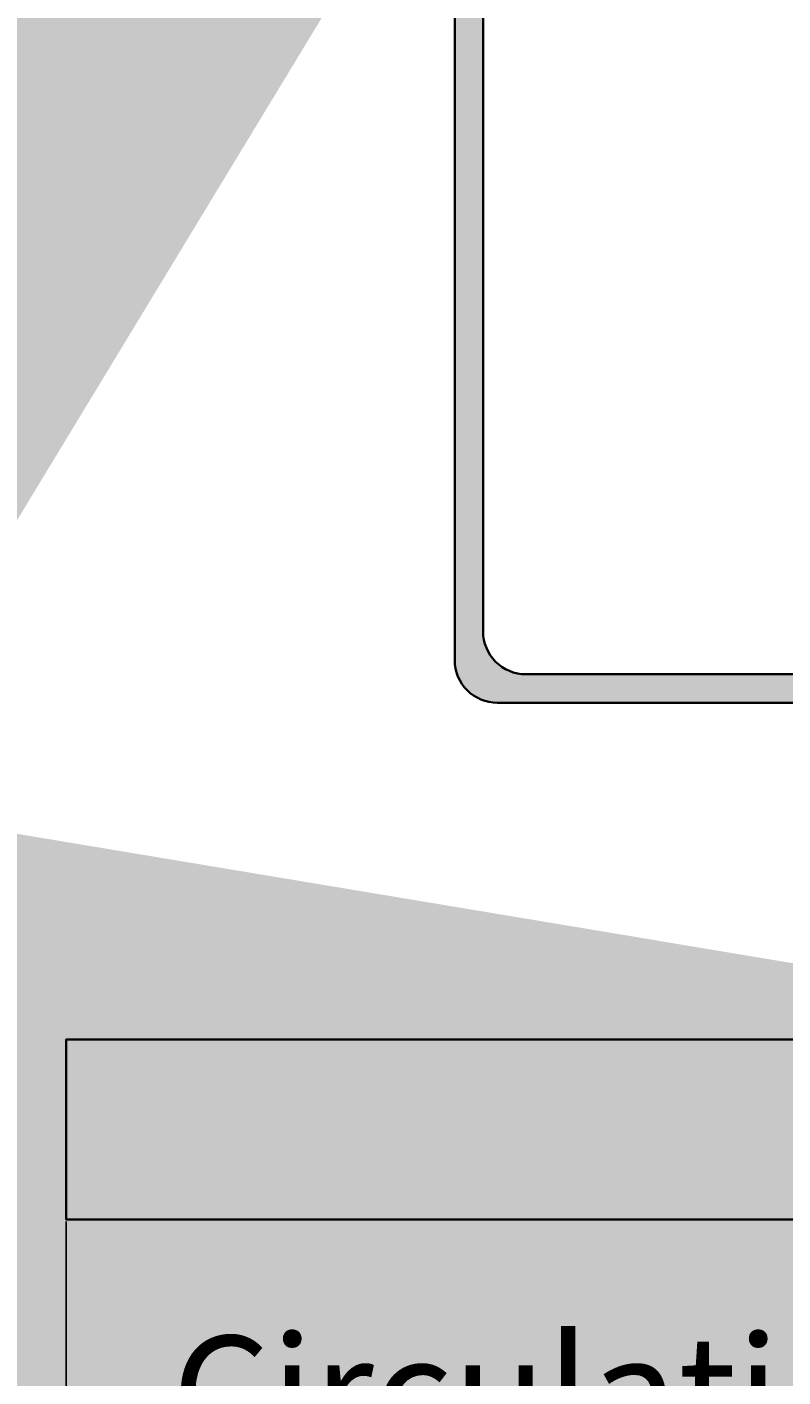
# Model space of a CAD drawing. Units: millimetres. Extents: x -22994 to 29398, y -19990 to 20176.
# Tile 9 of 135: x 5 to 32, y 5 to 52. Entities that reach past the tile are written whole.
import ezdxf
from ezdxf import colors
from ezdxf.entities.mleader import LeaderData, LeaderLine
from ezdxf.math import Vec2, Vec3

# ---------------------------------------------------------------- set-up
doc = ezdxf.new("R2010")
doc.units = ezdxf.units.MM
doc.header["$MEASUREMENT"] = 0
for name, color, linetype, lineweight in [('M-ANNO-TEXT', 7, 'Continuous', 25), ('M-DIMS', 2, 'Continuous', 18), ('M-EQPM-PATT', 7, 'Continuous', 18), ('M-PIPE', 7, 'Continuous', 35), ('S-FNDN', 7, 'Continuous', 35)]:
    doc.layers.add(name, color=color, linetype=linetype, lineweight=lineweight)
doc.styles.get("Standard").update_dxf_attribs({"font": 'arial.ttf'})
doc.dimstyles.get("Standard").update_dxf_attribs({"dimtxt": 0.18, "dimasz": 10000, "dimexe": 0.18, "dimexo": 0.0625, "dimgap": 0.09, "dimtad": 0, "dimtih": 1, "dimtoh": 1, "dimdec": 0, "dimzin": 0, "dimdsep": 46, "dimtxsty": 'Standard', "dimcen": 0.09, "dimadec": 0, "dimazin": 0, "dimtfac": 1, "dimtdec": 0, "dimtofl": 0, "dimtmove": 0, "dimatfit": 3, "dimfxl": 1, "dimtolj": 1, "dimtzin": 0, "dimlwd": 30, "dimarcsym": 0})

# ---------------------------------------------------------------- blocks, each defined once
blk = doc.blocks.new('*D2')
at = {"layer": 'Defpoints', "color": 0, "transparency": 16777216}
for p in [(6.677, 10.271), (290.852, 10.271), (290.852, -5.079)]:
    blk.add_point(p, dxfattribs=at)
at = {"layer": 'M-DIMS', "color": 0, "lineweight": -2, "transparency": 16777216}
for p, q in [((6.677, 10.209), (6.677, -5.259)), ((290.852, 10.209), (290.852, -5.259))]:
    blk.add_line(p, q, dxfattribs=at)
at = {"layer": 'M-DIMS', "color": 0, "lineweight": 30, "transparency": 16777216}
for p, q in [((-9993.323, -5.079), (-19993.323, -5.079)), ((10290.852, -5.079), (20290.852, -5.079))]:
    blk.add_line(p, q, dxfattribs=at)
at = {"layer": 'M-DIMS', "color": 0, "transparency": 16777216}
for points in [[(-9993.323, 1661.588), (-9993.323, -1671.745), (6.677, -5.079)], [(10290.852, 1661.588), (10290.852, -1671.745), (290.852, -5.079)]]:
    blk.add_solid(points, dxfattribs=at)
at = {"layer": 'M-DIMS', "color": 0, "transparency": 16777216, "insert": (148.765, -5.079), "char_height": 0.18, "attachment_point": 5}
blk.add_mtext('\\A1;284.2', dxfattribs=at)
blk = doc.blocks.new('*D3')
at = {"layer": 'Defpoints', "color": 0, "transparency": 16777216}
for p in [(110.265, 204.165), (110.265, 176.366), (95.833, 127.967)]:
    blk.add_point(p, dxfattribs=at)
at = {"layer": 'M-DIMS', "color": 0, "lineweight": 30, "transparency": 16777216}
for p, q in [((-9904.167, 204.165), (-19904.167, 204.165)), ((10110.265, 204.165), (20110.265, 204.165))]:
    blk.add_line(p, q, dxfattribs=at)
at = {"layer": 'M-DIMS', "color": 0, "lineweight": -2, "transparency": 16777216}
for p, q in [((95.833, 128.03), (95.833, 204.345)), ((110.265, 176.429), (110.265, 204.345))]:
    blk.add_line(p, q, dxfattribs=at)
at = {"layer": 'M-DIMS', "color": 0, "transparency": 16777216}
for points in [[(-9904.167, 1870.832), (-9904.167, -1462.501), (95.833, 204.165)], [(10110.265, 1870.832), (10110.265, -1462.501), (110.265, 204.165)]]:
    blk.add_solid(points, dxfattribs=at)
at = {"layer": 'M-DIMS', "color": 0, "transparency": 16777216, "insert": (103.049, 204.165), "char_height": 0.18, "attachment_point": 5}
blk.add_mtext('\\A1;14.432', dxfattribs=at)
blk = doc.blocks.new('*D4')
at = {"layer": 'Defpoints', "color": 0, "transparency": 16777216}
for p in [(116.265, 204.165), (110.265, 176.366), (116.265, 176.366)]:
    blk.add_point(p, dxfattribs=at)
at = {"layer": 'M-DIMS', "color": 0, "lineweight": 30, "transparency": 16777216}
for p, q in [((-9889.735, 204.165), (-19889.735, 204.165)), ((10116.265, 204.165), (20116.265, 204.165))]:
    blk.add_line(p, q, dxfattribs=at)
at = {"layer": 'M-DIMS', "color": 0, "lineweight": -2, "transparency": 16777216}
for p, q in [((110.265, 176.429), (110.265, 204.345)), ((116.265, 176.429), (116.265, 204.345))]:
    blk.add_line(p, q, dxfattribs=at)
at = {"layer": 'M-DIMS', "color": 0, "transparency": 16777216}
for points in [[(-9889.735, 1870.832), (-9889.735, -1462.501), (110.265, 204.165)], [(10116.265, 1870.832), (10116.265, -1462.501), (116.265, 204.165)]]:
    blk.add_solid(points, dxfattribs=at)
at = {"layer": 'M-DIMS', "color": 0, "transparency": 16777216, "insert": (113.265, 204.165), "char_height": 0.18, "attachment_point": 5}
blk.add_mtext('\\A1;6', dxfattribs=at)
blk = doc.blocks.new('*D5')
at = {"layer": 'Defpoints', "color": 0, "transparency": 16777216}
for p in [(181.265, 204.165), (116.265, 176.366), (181.265, 176.366)]:
    blk.add_point(p, dxfattribs=at)
at = {"layer": 'M-DIMS', "color": 0, "lineweight": 30, "transparency": 16777216}
for p, q in [((-9883.735, 204.165), (-19883.735, 204.165)), ((10181.265, 204.165), (20181.265, 204.165))]:
    blk.add_line(p, q, dxfattribs=at)
at = {"layer": 'M-DIMS', "color": 0, "lineweight": -2, "transparency": 16777216}
for p, q in [((116.265, 176.429), (116.265, 204.345)), ((181.265, 176.429), (181.265, 204.345))]:
    blk.add_line(p, q, dxfattribs=at)
at = {"layer": 'M-DIMS', "color": 0, "transparency": 16777216}
for points in [[(-9883.735, 1870.832), (-9883.735, -1462.501), (116.265, 204.165)], [(10181.265, 1870.832), (10181.265, -1462.501), (181.265, 204.165)]]:
    blk.add_solid(points, dxfattribs=at)
at = {"layer": 'M-DIMS', "color": 0, "transparency": 16777216, "insert": (148.765, 204.165), "char_height": 0.18, "attachment_point": 5}
blk.add_mtext('\\A1;65', dxfattribs=at)
blk = doc.blocks.new('*D6')
at = {"layer": 'Defpoints', "color": 0, "transparency": 16777216}
for p in [(187.265, 204.165), (181.265, 176.366), (187.265, 176.366)]:
    blk.add_point(p, dxfattribs=at)
at = {"layer": 'M-DIMS', "color": 0, "lineweight": 30, "transparency": 16777216}
for p, q in [((-9818.735, 204.165), (-19818.735, 204.165)), ((10187.265, 204.165), (20187.265, 204.165))]:
    blk.add_line(p, q, dxfattribs=at)
at = {"layer": 'M-DIMS', "color": 0, "lineweight": -2, "transparency": 16777216}
for p, q in [((181.265, 176.429), (181.265, 204.345)), ((187.265, 176.429), (187.265, 204.345))]:
    blk.add_line(p, q, dxfattribs=at)
at = {"layer": 'M-DIMS', "color": 0, "transparency": 16777216}
for points in [[(-9818.735, 1870.832), (-9818.735, -1462.501), (181.265, 204.165)], [(10187.265, 1870.832), (10187.265, -1462.501), (187.265, 204.165)]]:
    blk.add_solid(points, dxfattribs=at)
at = {"layer": 'M-DIMS', "color": 0, "transparency": 16777216, "insert": (184.265, 204.165), "char_height": 0.18, "attachment_point": 5}
blk.add_mtext('\\A1;6', dxfattribs=at)
blk = doc.blocks.new('*D7')
at = {"layer": 'Defpoints', "color": 0, "transparency": 16777216}
for p in [(201.697, 204.165), (187.265, 176.366), (201.697, 127.967)]:
    blk.add_point(p, dxfattribs=at)
at = {"layer": 'M-DIMS', "color": 0, "lineweight": 30, "transparency": 16777216}
for p, q in [((-9812.735, 204.165), (-19812.735, 204.165)), ((10201.697, 204.165), (20201.697, 204.165))]:
    blk.add_line(p, q, dxfattribs=at)
at = {"layer": 'M-DIMS', "color": 0, "lineweight": -2, "transparency": 16777216}
for p, q in [((187.265, 176.429), (187.265, 204.345)), ((201.697, 128.03), (201.697, 204.345))]:
    blk.add_line(p, q, dxfattribs=at)
at = {"layer": 'M-DIMS', "color": 0, "transparency": 16777216}
for points in [[(-9812.735, 1870.832), (-9812.735, -1462.501), (187.265, 204.165)], [(10201.697, 1870.832), (10201.697, -1462.501), (201.697, 204.165)]]:
    blk.add_solid(points, dxfattribs=at)
at = {"layer": 'M-DIMS', "color": 0, "transparency": 16777216, "insert": (194.481, 204.165), "char_height": 0.18, "attachment_point": 5}
blk.add_mtext('\\A1;14.432', dxfattribs=at)
blk = doc.blocks.new('*D8')
at = {"layer": 'Defpoints', "color": 0, "transparency": 16777216}
for p in [(227.648, 204.165), (227.648, 146.73), (201.697, 127.967)]:
    blk.add_point(p, dxfattribs=at)
at = {"layer": 'M-DIMS', "color": 0, "lineweight": 30, "transparency": 16777216}
for p, q in [((-9798.303, 204.165), (-19798.303, 204.165)), ((10227.648, 204.165), (20227.648, 204.165))]:
    blk.add_line(p, q, dxfattribs=at)
at = {"layer": 'M-DIMS', "color": 0, "lineweight": -2, "transparency": 16777216}
for p, q in [((201.697, 128.03), (201.697, 204.345)), ((227.648, 146.792), (227.648, 204.345))]:
    blk.add_line(p, q, dxfattribs=at)
at = {"layer": 'M-DIMS', "color": 0, "transparency": 16777216}
for points in [[(-9798.303, 1870.832), (-9798.303, -1462.501), (201.697, 204.165)], [(10227.648, 1870.832), (10227.648, -1462.501), (227.648, 204.165)]]:
    blk.add_solid(points, dxfattribs=at)
at = {"layer": 'M-DIMS', "color": 0, "transparency": 16777216, "insert": (214.673, 204.165), "char_height": 0.18, "attachment_point": 5}
blk.add_mtext('\\A1;25.95', dxfattribs=at)
blk = doc.blocks.new('*D9')
at = {"layer": 'Defpoints', "color": 0, "transparency": 16777216}
for p in [(187.265, 176.366), (306.202, 176.366), (290.852, 10.271)]:
    blk.add_point(p, dxfattribs=at)
at = {"layer": 'M-DIMS', "color": 0, "lineweight": 30, "transparency": 16777216}
for p, q in [((306.202, 10176.366), (306.202, 20176.366)), ((306.202, -9989.729), (306.202, -19989.729))]:
    blk.add_line(p, q, dxfattribs=at)
at = {"layer": 'M-DIMS', "color": 0, "lineweight": -2, "transparency": 16777216}
for p, q in [((187.327, 176.366), (306.382, 176.366)), ((290.915, 10.271), (306.382, 10.271))]:
    blk.add_line(p, q, dxfattribs=at)
at = {"layer": 'M-DIMS', "color": 0, "transparency": 16777216}
for points in [[(-1360.465, 10176.366), (1972.869, 10176.366), (306.202, 176.366)], [(-1360.465, -9989.729), (1972.869, -9989.729), (306.202, 10.271)]]:
    blk.add_solid(points, dxfattribs=at)
at = {"layer": 'M-DIMS', "color": 0, "transparency": 16777216, "insert": (306.202, 93.319), "char_height": 0.18, "attachment_point": 5}
blk.add_mtext('\\A1;166.1', dxfattribs=at)
blk = doc.blocks.new('*D10')
at = {"layer": 'Defpoints', "color": 0, "transparency": 16777216}
for p in [(125.65, 136.071), (133.346, 136.071), (133.346, -5.079)]:
    blk.add_point(p, dxfattribs=at)
at = {"layer": 'M-DIMS', "color": 0, "lineweight": -2, "transparency": 16777216}
for p, q in [((125.65, 136.009), (125.65, -5.259)), ((133.346, 136.009), (133.346, -5.259))]:
    blk.add_line(p, q, dxfattribs=at)
at = {"layer": 'M-DIMS', "color": 0, "lineweight": 30, "transparency": 16777216}
for p, q in [((-9874.35, -5.079), (-19874.35, -5.079)), ((10133.346, -5.079), (20133.346, -5.079))]:
    blk.add_line(p, q, dxfattribs=at)
at = {"layer": 'M-DIMS', "color": 0, "transparency": 16777216}
for points in [[(-9874.35, 1661.588), (-9874.35, -1671.745), (125.65, -5.079)], [(10133.346, 1661.588), (10133.346, -1671.745), (133.346, -5.079)]]:
    blk.add_solid(points, dxfattribs=at)
at = {"layer": 'M-DIMS', "color": 0, "transparency": 16777216, "insert": (129.498, -5.079), "char_height": 0.18, "attachment_point": 5}
blk.add_mtext('\\A1;7.696', dxfattribs=at)
blk = doc.blocks.new('*D11')
at = {"layer": 'Defpoints', "color": 0, "transparency": 16777216}
for p in [(133.346, 136.071), (135.65, 136.071), (135.65, -5.079)]:
    blk.add_point(p, dxfattribs=at)
at = {"layer": 'M-DIMS', "color": 0, "lineweight": -2, "transparency": 16777216}
for p, q in [((133.346, 136.009), (133.346, -5.259)), ((135.65, 136.009), (135.65, -5.259))]:
    blk.add_line(p, q, dxfattribs=at)
at = {"layer": 'M-DIMS', "color": 0, "lineweight": 30, "transparency": 16777216}
for p, q in [((-9866.654, -5.079), (-19866.654, -5.079)), ((10135.65, -5.079), (20135.65, -5.079))]:
    blk.add_line(p, q, dxfattribs=at)
at = {"layer": 'M-DIMS', "color": 0, "transparency": 16777216}
for points in [[(-9866.654, 1661.588), (-9866.654, -1671.745), (133.346, -5.079)], [(10135.65, 1661.588), (10135.65, -1671.745), (135.65, -5.079)]]:
    blk.add_solid(points, dxfattribs=at)
at = {"layer": 'M-DIMS', "color": 0, "transparency": 16777216, "insert": (134.498, -5.079), "char_height": 0.18, "attachment_point": 5}
blk.add_mtext('\\A1;2.304', dxfattribs=at)
blk = doc.blocks.new('*D12')
at = {"layer": 'Defpoints', "color": 0, "transparency": 16777216}
for p in [(135.65, 136.071), (145.65, 136.071), (145.65, -5.079)]:
    blk.add_point(p, dxfattribs=at)
at = {"layer": 'M-DIMS', "color": 0, "lineweight": -2, "transparency": 16777216}
for p, q in [((135.65, 136.009), (135.65, -5.259)), ((145.65, 136.009), (145.65, -5.259))]:
    blk.add_line(p, q, dxfattribs=at)
at = {"layer": 'M-DIMS', "color": 0, "lineweight": 30, "transparency": 16777216}
for p, q in [((-9864.35, -5.079), (-19864.35, -5.079)), ((10145.65, -5.079), (20145.65, -5.079))]:
    blk.add_line(p, q, dxfattribs=at)
at = {"layer": 'M-DIMS', "color": 0, "transparency": 16777216}
for points in [[(-9864.35, 1661.588), (-9864.35, -1671.745), (135.65, -5.079)], [(10145.65, 1661.588), (10145.65, -1671.745), (145.65, -5.079)]]:
    blk.add_solid(points, dxfattribs=at)
at = {"layer": 'M-DIMS', "color": 0, "transparency": 16777216, "insert": (140.65, -5.079), "char_height": 0.18, "attachment_point": 5}
blk.add_mtext('\\A1;10', dxfattribs=at)
blk = doc.blocks.new('*D13')
at = {"layer": 'Defpoints', "color": 0, "transparency": 16777216}
for p in [(145.65, 136.071), (155.65, 136.071), (155.65, -5.079)]:
    blk.add_point(p, dxfattribs=at)
at = {"layer": 'M-DIMS', "color": 0, "lineweight": -2, "transparency": 16777216}
for p, q in [((145.65, 136.009), (145.65, -5.259)), ((155.65, 136.009), (155.65, -5.259))]:
    blk.add_line(p, q, dxfattribs=at)
at = {"layer": 'M-DIMS', "color": 0, "lineweight": 30, "transparency": 16777216}
for p, q in [((-9854.35, -5.079), (-19854.35, -5.079)), ((10155.65, -5.079), (20155.65, -5.079))]:
    blk.add_line(p, q, dxfattribs=at)
at = {"layer": 'M-DIMS', "color": 0, "transparency": 16777216}
for points in [[(-9854.35, 1661.588), (-9854.35, -1671.745), (145.65, -5.079)], [(10155.65, 1661.588), (10155.65, -1671.745), (155.65, -5.079)]]:
    blk.add_solid(points, dxfattribs=at)
at = {"layer": 'M-DIMS', "color": 0, "transparency": 16777216, "insert": (150.65, -5.079), "char_height": 0.18, "attachment_point": 5}
blk.add_mtext('\\A1;10', dxfattribs=at)
blk = doc.blocks.new('*D14')
at = {"layer": 'Defpoints', "color": 0, "transparency": 16777216}
for p in [(155.65, 136.071), (165.65, 136.071), (165.65, -5.079)]:
    blk.add_point(p, dxfattribs=at)
at = {"layer": 'M-DIMS', "color": 0, "lineweight": -2, "transparency": 16777216}
for p, q in [((155.65, 136.009), (155.65, -5.259)), ((165.65, 136.009), (165.65, -5.259))]:
    blk.add_line(p, q, dxfattribs=at)
at = {"layer": 'M-DIMS', "color": 0, "lineweight": 30, "transparency": 16777216}
for p, q in [((-9844.35, -5.079), (-19844.35, -5.079)), ((10165.65, -5.079), (20165.65, -5.079))]:
    blk.add_line(p, q, dxfattribs=at)
at = {"layer": 'M-DIMS', "color": 0, "transparency": 16777216}
for points in [[(-9844.35, 1661.588), (-9844.35, -1671.745), (155.65, -5.079)], [(10165.65, 1661.588), (10165.65, -1671.745), (165.65, -5.079)]]:
    blk.add_solid(points, dxfattribs=at)
at = {"layer": 'M-DIMS', "color": 0, "transparency": 16777216, "insert": (160.65, -5.079), "char_height": 0.18, "attachment_point": 5}
blk.add_mtext('\\A1;10', dxfattribs=at)
blk = doc.blocks.new('*D15')
at = {"layer": 'Defpoints', "color": 0, "transparency": 16777216}
for p in [(173.346, 154.788), (173.346, 136.071), (306.202, 136.071)]:
    blk.add_point(p, dxfattribs=at)
at = {"layer": 'M-DIMS', "color": 0, "lineweight": 30, "transparency": 16777216}
for p, q in [((306.202, 10154.788), (306.202, 20154.788)), ((306.202, -9863.929), (306.202, -19863.929))]:
    blk.add_line(p, q, dxfattribs=at)
at = {"layer": 'M-DIMS', "color": 0, "lineweight": -2, "transparency": 16777216}
for p, q in [((173.408, 154.788), (306.382, 154.788)), ((173.408, 136.071), (306.382, 136.071))]:
    blk.add_line(p, q, dxfattribs=at)
at = {"layer": 'M-DIMS', "color": 0, "transparency": 16777216}
for points in [[(-1360.465, 10154.788), (1972.869, 10154.788), (306.202, 154.788)], [(-1360.465, -9863.929), (1972.869, -9863.929), (306.202, 136.071)]]:
    blk.add_solid(points, dxfattribs=at)
at = {"layer": 'M-DIMS', "color": 0, "transparency": 16777216, "insert": (306.202, 145.43), "char_height": 0.18, "attachment_point": 5}
blk.add_mtext('\\A1;18.717', dxfattribs=at)
blk = doc.blocks.new('*D16')
at = {"layer": 'Defpoints', "color": 0, "transparency": 16777216}
for p in [(120.17, 204.165), (110.466, 48.035), (120.17, 48.035)]:
    blk.add_point(p, dxfattribs=at)
at = {"layer": 'M-DIMS', "color": 0, "lineweight": 30, "transparency": 16777216}
for p, q in [((-9889.534, 204.165), (-19889.534, 204.165)), ((10120.17, 204.165), (20120.17, 204.165))]:
    blk.add_line(p, q, dxfattribs=at)
at = {"layer": 'M-DIMS', "color": 0, "lineweight": -2, "transparency": 16777216}
for p, q in [((110.466, 48.097), (110.466, 204.345)), ((120.17, 48.097), (120.17, 204.345))]:
    blk.add_line(p, q, dxfattribs=at)
at = {"layer": 'M-DIMS', "color": 0, "transparency": 16777216}
for points in [[(-9889.534, 1870.832), (-9889.534, -1462.501), (110.466, 204.165)], [(10120.17, 1870.832), (10120.17, -1462.501), (120.17, 204.165)]]:
    blk.add_solid(points, dxfattribs=at)
at = {"layer": 'M-DIMS', "color": 0, "transparency": 16777216, "insert": (115.318, 204.165), "char_height": 0.18, "attachment_point": 5}
blk.add_mtext('\\A1;9.704', dxfattribs=at)
blk = doc.blocks.new('*D17')
at = {"layer": 'Defpoints', "color": 0, "transparency": 16777216}
for p in [(126.17, 204.165), (120.17, 48.035), (126.17, 48.035)]:
    blk.add_point(p, dxfattribs=at)
at = {"layer": 'M-DIMS', "color": 0, "lineweight": 30, "transparency": 16777216}
for p, q in [((-9879.83, 204.165), (-19879.83, 204.165)), ((10126.17, 204.165), (20126.17, 204.165))]:
    blk.add_line(p, q, dxfattribs=at)
at = {"layer": 'M-DIMS', "color": 0, "lineweight": -2, "transparency": 16777216}
for p, q in [((120.17, 48.097), (120.17, 204.345)), ((126.17, 48.097), (126.17, 204.345))]:
    blk.add_line(p, q, dxfattribs=at)
at = {"layer": 'M-DIMS', "color": 0, "transparency": 16777216}
for points in [[(-9879.83, 1870.832), (-9879.83, -1462.501), (120.17, 204.165)], [(10126.17, 1870.832), (10126.17, -1462.501), (126.17, 204.165)]]:
    blk.add_solid(points, dxfattribs=at)
at = {"layer": 'M-DIMS', "color": 0, "transparency": 16777216, "insert": (123.17, 204.165), "char_height": 0.18, "attachment_point": 5}
blk.add_mtext('\\A1;6', dxfattribs=at)
blk = doc.blocks.new('*D18')
at = {"layer": 'Defpoints', "color": 0, "transparency": 16777216}
for p in [(132.17, 204.165), (126.17, 48.035), (132.17, 48.035)]:
    blk.add_point(p, dxfattribs=at)
at = {"layer": 'M-DIMS', "color": 0, "lineweight": 30, "transparency": 16777216}
for p, q in [((-9873.83, 204.165), (-19873.83, 204.165)), ((10132.17, 204.165), (20132.17, 204.165))]:
    blk.add_line(p, q, dxfattribs=at)
at = {"layer": 'M-DIMS', "color": 0, "lineweight": -2, "transparency": 16777216}
for p, q in [((126.17, 48.097), (126.17, 204.345)), ((132.17, 48.097), (132.17, 204.345))]:
    blk.add_line(p, q, dxfattribs=at)
at = {"layer": 'M-DIMS', "color": 0, "transparency": 16777216}
for points in [[(-9873.83, 1870.832), (-9873.83, -1462.501), (126.17, 204.165)], [(10132.17, 1870.832), (10132.17, -1462.501), (132.17, 204.165)]]:
    blk.add_solid(points, dxfattribs=at)
at = {"layer": 'M-DIMS', "color": 0, "transparency": 16777216, "insert": (129.17, 204.165), "char_height": 0.18, "attachment_point": 5}
blk.add_mtext('\\A1;6', dxfattribs=at)
blk = doc.blocks.new('*D19')
at = {"layer": 'Defpoints', "color": 0, "transparency": 16777216}
for p in [(138.17, 204.165), (132.17, 48.035), (138.17, 48.035)]:
    blk.add_point(p, dxfattribs=at)
at = {"layer": 'M-DIMS', "color": 0, "lineweight": 30, "transparency": 16777216}
for p, q in [((-9867.83, 204.165), (-19867.83, 204.165)), ((10138.17, 204.165), (20138.17, 204.165))]:
    blk.add_line(p, q, dxfattribs=at)
at = {"layer": 'M-DIMS', "color": 0, "lineweight": -2, "transparency": 16777216}
for p, q in [((132.17, 48.097), (132.17, 204.345)), ((138.17, 48.097), (138.17, 204.345))]:
    blk.add_line(p, q, dxfattribs=at)
at = {"layer": 'M-DIMS', "color": 0, "transparency": 16777216}
for points in [[(-9867.83, 1870.832), (-9867.83, -1462.501), (132.17, 204.165)], [(10138.17, 1870.832), (10138.17, -1462.501), (138.17, 204.165)]]:
    blk.add_solid(points, dxfattribs=at)
at = {"layer": 'M-DIMS', "color": 0, "transparency": 16777216, "insert": (135.17, 204.165), "char_height": 0.18, "attachment_point": 5}
blk.add_mtext('\\A1;6', dxfattribs=at)
blk = doc.blocks.new('*D20')
at = {"layer": 'Defpoints', "color": 0, "transparency": 16777216}
for p in [(144.17, 204.165), (138.17, 48.035), (144.17, 48.035)]:
    blk.add_point(p, dxfattribs=at)
at = {"layer": 'M-DIMS', "color": 0, "lineweight": 30, "transparency": 16777216}
for p, q in [((-9861.83, 204.165), (-19861.83, 204.165)), ((10144.17, 204.165), (20144.17, 204.165))]:
    blk.add_line(p, q, dxfattribs=at)
at = {"layer": 'M-DIMS', "color": 0, "lineweight": -2, "transparency": 16777216}
for p, q in [((138.17, 48.097), (138.17, 204.345)), ((144.17, 48.097), (144.17, 204.345))]:
    blk.add_line(p, q, dxfattribs=at)
at = {"layer": 'M-DIMS', "color": 0, "transparency": 16777216}
for points in [[(-9861.83, 1870.832), (-9861.83, -1462.501), (138.17, 204.165)], [(10144.17, 1870.832), (10144.17, -1462.501), (144.17, 204.165)]]:
    blk.add_solid(points, dxfattribs=at)
at = {"layer": 'M-DIMS', "color": 0, "transparency": 16777216, "insert": (141.17, 204.165), "char_height": 0.18, "attachment_point": 5}
blk.add_mtext('\\A1;6', dxfattribs=at)
blk = doc.blocks.new('*D21')
at = {"layer": 'Defpoints', "color": 0, "transparency": 16777216}
for p in [(149.116, 204.165), (144.17, 48.035), (149.116, 48.035)]:
    blk.add_point(p, dxfattribs=at)
at = {"layer": 'M-DIMS', "color": 0, "lineweight": 30, "transparency": 16777216}
for p, q in [((-9855.83, 204.165), (-19855.83, 204.165)), ((10149.116, 204.165), (20149.116, 204.165))]:
    blk.add_line(p, q, dxfattribs=at)
at = {"layer": 'M-DIMS', "color": 0, "lineweight": -2, "transparency": 16777216}
for p, q in [((144.17, 48.097), (144.17, 204.345)), ((149.116, 48.097), (149.116, 204.345))]:
    blk.add_line(p, q, dxfattribs=at)
at = {"layer": 'M-DIMS', "color": 0, "transparency": 16777216}
for points in [[(-9855.83, 1870.832), (-9855.83, -1462.501), (144.17, 204.165)], [(10149.116, 1870.832), (10149.116, -1462.501), (149.116, 204.165)]]:
    blk.add_solid(points, dxfattribs=at)
at = {"layer": 'M-DIMS', "color": 0, "transparency": 16777216, "insert": (146.643, 204.165), "char_height": 0.18, "attachment_point": 5}
blk.add_mtext('\\A1;4.945', dxfattribs=at)
blk = doc.blocks.new('*D22')
at = {"layer": 'Defpoints', "color": 0, "transparency": 16777216}
for p in [(149.116, 30.99), (155.116, 30.99), (155.116, -5.079)]:
    blk.add_point(p, dxfattribs=at)
at = {"layer": 'M-DIMS', "color": 0, "lineweight": -2, "transparency": 16777216}
for p, q in [((149.116, 30.927), (149.116, -5.259)), ((155.116, 30.927), (155.116, -5.259))]:
    blk.add_line(p, q, dxfattribs=at)
at = {"layer": 'M-DIMS', "color": 0, "lineweight": 30, "transparency": 16777216}
for p, q in [((-9850.884, -5.079), (-19850.884, -5.079)), ((10155.116, -5.079), (20155.116, -5.079))]:
    blk.add_line(p, q, dxfattribs=at)
at = {"layer": 'M-DIMS', "color": 0, "transparency": 16777216}
for points in [[(-9850.884, 1661.588), (-9850.884, -1671.745), (149.116, -5.079)], [(10155.116, 1661.588), (10155.116, -1671.745), (155.116, -5.079)]]:
    blk.add_solid(points, dxfattribs=at)
at = {"layer": 'M-DIMS', "color": 0, "transparency": 16777216, "insert": (152.116, -5.079), "char_height": 0.18, "attachment_point": 5}
blk.add_mtext('\\A1;6', dxfattribs=at)
blk = doc.blocks.new('*D23')
at = {"layer": 'Defpoints', "color": 0, "transparency": 16777216}
for p in [(155.116, 30.99), (161.116, 30.99), (161.116, -5.079)]:
    blk.add_point(p, dxfattribs=at)
at = {"layer": 'M-DIMS', "color": 0, "lineweight": -2, "transparency": 16777216}
for p, q in [((155.116, 30.927), (155.116, -5.259)), ((161.116, 30.927), (161.116, -5.259))]:
    blk.add_line(p, q, dxfattribs=at)
at = {"layer": 'M-DIMS', "color": 0, "lineweight": 30, "transparency": 16777216}
for p, q in [((-9844.884, -5.079), (-19844.884, -5.079)), ((10161.116, -5.079), (20161.116, -5.079))]:
    blk.add_line(p, q, dxfattribs=at)
at = {"layer": 'M-DIMS', "color": 0, "transparency": 16777216}
for points in [[(-9844.884, 1661.588), (-9844.884, -1671.745), (155.116, -5.079)], [(10161.116, 1661.588), (10161.116, -1671.745), (161.116, -5.079)]]:
    blk.add_solid(points, dxfattribs=at)
at = {"layer": 'M-DIMS', "color": 0, "transparency": 16777216, "insert": (158.116, -5.079), "char_height": 0.18, "attachment_point": 5}
blk.add_mtext('\\A1;6', dxfattribs=at)
blk = doc.blocks.new('*D24')
at = {"layer": 'Defpoints', "color": 0, "transparency": 16777216}
for p in [(161.116, 30.99), (166.439, 30.99), (166.439, -5.079)]:
    blk.add_point(p, dxfattribs=at)
at = {"layer": 'M-DIMS', "color": 0, "lineweight": -2, "transparency": 16777216}
for p, q in [((161.116, 30.927), (161.116, -5.259)), ((166.439, 30.927), (166.439, -5.259))]:
    blk.add_line(p, q, dxfattribs=at)
at = {"layer": 'M-DIMS', "color": 0, "lineweight": 30, "transparency": 16777216}
for p, q in [((-9838.884, -5.079), (-19838.884, -5.079)), ((10166.439, -5.079), (20166.439, -5.079))]:
    blk.add_line(p, q, dxfattribs=at)
at = {"layer": 'M-DIMS', "color": 0, "transparency": 16777216}
for points in [[(-9838.884, 1661.588), (-9838.884, -1671.745), (161.116, -5.079)], [(10166.439, 1661.588), (10166.439, -1671.745), (166.439, -5.079)]]:
    blk.add_solid(points, dxfattribs=at)
at = {"layer": 'M-DIMS', "color": 0, "transparency": 16777216, "insert": (163.777, -5.079), "char_height": 0.18, "attachment_point": 5}
blk.add_mtext('\\A1;5.323', dxfattribs=at)
blk = doc.blocks.new('*D25')
at = {"layer": 'Defpoints', "color": 0, "transparency": 16777216}
for p in [(166.439, 30.99), (172.439, 30.99), (172.439, -5.079)]:
    blk.add_point(p, dxfattribs=at)
at = {"layer": 'M-DIMS', "color": 0, "lineweight": -2, "transparency": 16777216}
for p, q in [((166.439, 30.927), (166.439, -5.259)), ((172.439, 30.927), (172.439, -5.259))]:
    blk.add_line(p, q, dxfattribs=at)
at = {"layer": 'M-DIMS', "color": 0, "lineweight": 30, "transparency": 16777216}
for p, q in [((-9833.561, -5.079), (-19833.561, -5.079)), ((10172.439, -5.079), (20172.439, -5.079))]:
    blk.add_line(p, q, dxfattribs=at)
at = {"layer": 'M-DIMS', "color": 0, "transparency": 16777216}
for points in [[(-9833.561, 1661.588), (-9833.561, -1671.745), (166.439, -5.079)], [(10172.439, 1661.588), (10172.439, -1671.745), (172.439, -5.079)]]:
    blk.add_solid(points, dxfattribs=at)
at = {"layer": 'M-DIMS', "color": 0, "transparency": 16777216, "insert": (169.439, -5.079), "char_height": 0.18, "attachment_point": 5}
blk.add_mtext('\\A1;6', dxfattribs=at)
blk = doc.blocks.new('*D26')
at = {"layer": 'Defpoints', "color": 0, "transparency": 16777216}
for p in [(172.439, 30.99), (178.439, 30.99), (178.439, -5.079)]:
    blk.add_point(p, dxfattribs=at)
at = {"layer": 'M-DIMS', "color": 0, "lineweight": -2, "transparency": 16777216}
for p, q in [((172.439, 30.927), (172.439, -5.259)), ((178.439, 30.927), (178.439, -5.259))]:
    blk.add_line(p, q, dxfattribs=at)
at = {"layer": 'M-DIMS', "color": 0, "lineweight": 30, "transparency": 16777216}
for p, q in [((-9827.561, -5.079), (-19827.561, -5.079)), ((10178.439, -5.079), (20178.439, -5.079))]:
    blk.add_line(p, q, dxfattribs=at)
at = {"layer": 'M-DIMS', "color": 0, "transparency": 16777216}
for points in [[(-9827.561, 1661.588), (-9827.561, -1671.745), (172.439, -5.079)], [(10178.439, 1661.588), (10178.439, -1671.745), (178.439, -5.079)]]:
    blk.add_solid(points, dxfattribs=at)
at = {"layer": 'M-DIMS', "color": 0, "transparency": 16777216, "insert": (175.439, -5.079), "char_height": 0.18, "attachment_point": 5}
blk.add_mtext('\\A1;6', dxfattribs=at)
blk = doc.blocks.new('*D27')
at = {"layer": 'Defpoints', "color": 0, "transparency": 16777216}
for p in [(178.439, 30.99), (188.117, 30.99), (188.117, -5.079)]:
    blk.add_point(p, dxfattribs=at)
at = {"layer": 'M-DIMS', "color": 0, "lineweight": -2, "transparency": 16777216}
for p, q in [((178.439, 30.927), (178.439, -5.259)), ((188.117, 30.927), (188.117, -5.259))]:
    blk.add_line(p, q, dxfattribs=at)
at = {"layer": 'M-DIMS', "color": 0, "lineweight": 30, "transparency": 16777216}
for p, q in [((-9821.561, -5.079), (-19821.561, -5.079)), ((10188.117, -5.079), (20188.117, -5.079))]:
    blk.add_line(p, q, dxfattribs=at)
at = {"layer": 'M-DIMS', "color": 0, "transparency": 16777216}
for points in [[(-9821.561, 1661.588), (-9821.561, -1671.745), (178.439, -5.079)], [(10188.117, 1661.588), (10188.117, -1671.745), (188.117, -5.079)]]:
    blk.add_solid(points, dxfattribs=at)
at = {"layer": 'M-DIMS', "color": 0, "transparency": 16777216, "insert": (183.278, -5.079), "char_height": 0.18, "attachment_point": 5}
blk.add_mtext('\\A1;9.679', dxfattribs=at)
blk = doc.blocks.new('*D28')
at = {"layer": 'Defpoints', "color": 0, "transparency": 16777216}
for p in [(188.117, 48.035), (306.202, 48.035), (188.117, 30.99)]:
    blk.add_point(p, dxfattribs=at)
at = {"layer": 'M-DIMS', "color": 0, "lineweight": 30, "transparency": 16777216}
for p, q in [((306.202, 10048.035), (306.202, 20048.035)), ((306.202, -9969.01), (306.202, -19969.01))]:
    blk.add_line(p, q, dxfattribs=at)
at = {"layer": 'M-DIMS', "color": 0, "lineweight": -2, "transparency": 16777216}
for p, q in [((188.18, 48.035), (306.382, 48.035)), ((188.18, 30.99), (306.382, 30.99))]:
    blk.add_line(p, q, dxfattribs=at)
at = {"layer": 'M-DIMS', "color": 0, "transparency": 16777216}
for points in [[(-1360.465, 10048.035), (1972.869, 10048.035), (306.202, 48.035)], [(-1360.465, -9969.01), (1972.869, -9969.01), (306.202, 30.99)]]:
    blk.add_solid(points, dxfattribs=at)
at = {"layer": 'M-DIMS', "color": 0, "transparency": 16777216, "insert": (306.202, 39.512), "char_height": 0.18, "attachment_point": 5}
blk.add_mtext('\\A1;17.045', dxfattribs=at)
blk = doc.blocks.new('*D32')
at = {"layer": 'Defpoints', "color": 0, "transparency": 16777216}
for p in [(57.164, 118.614), (52.413, 113.093)]:
    blk.add_point(p, dxfattribs=at)
at = {"layer": 'M-DIMS', "color": 0, "lineweight": -2, "transparency": 16777216}
for p, q in [((57.164, 118.524), (57.164, 118.704)), ((57.074, 118.614), (57.254, 118.614))]:
    blk.add_line(p, q, dxfattribs=at)
at = {"layer": 'M-DIMS', "color": 0, "lineweight": 30, "transparency": 16777216}
for p, q in [((-12992.534, -15047.031), (-6470.06, -7466.969)), ((-22992.534, -15047.031), (-12992.534, -15047.031))]:
    blk.add_line(p, q, dxfattribs=at)
at = {"layer": 'M-DIMS', "color": 0, "transparency": 16777216}
blk.add_solid([(-7733.404, -6379.89), (-5206.717, -8554.048), (52.413, 113.093)], dxfattribs=at)
at = {"layer": 'M-DIMS', "color": 0, "transparency": 16777216, "insert": (-22993.208, -15047.031), "char_height": 0.18, "attachment_point": 5}
blk.add_mtext('\\A1;2X R7.284', dxfattribs=at)
blk = doc.blocks.new('*D36')
at = {"layer": 'Defpoints', "color": 0, "transparency": 16777216}
for p in [(46.39, 31.303), (46.387, 26.593)]:
    blk.add_point(p, dxfattribs=at)
at = {"layer": 'M-DIMS', "color": 0, "lineweight": 30, "transparency": 16777216}
for p, q in [((57.15, 20031.301), (51.77, 10031.302)), ((10057.15, 20031.301), (57.15, 20031.301))]:
    blk.add_line(p, q, dxfattribs=at)
at = {"layer": 'M-DIMS', "color": 0, "lineweight": -2, "transparency": 16777216}
for p, q in [((46.389, 28.858), (46.389, 29.038)), ((46.299, 28.948), (46.479, 28.948))]:
    blk.add_line(p, q, dxfattribs=at)
at = {"layer": 'M-DIMS', "color": 0, "transparency": 16777216}
blk.add_solid([(-1614.896, 10032.199), (1718.436, 10030.405), (46.39, 31.303)], dxfattribs=at)
at = {"layer": 'M-DIMS', "color": 0, "transparency": 16777216, "insert": (10057.554, 20031.301), "char_height": 0.18, "attachment_point": 5}
blk.add_mtext('\\A1;∅4.71', dxfattribs=at)

msp = doc.modelspace()

# ---------------------------------------------------------------- hatches: boundary and pattern name
at = {"layer": 'M-EQPM-PATT'}
h = msp.add_hatch(color=256, dxfattribs=at)
h.set_gradient(color1=(16, 86, 137), color2=(39, 118, 187), tint=1, name='CYLINDER')
h.paths.add_polyline_path([(22.8402, 76.5922), (37.2457, 76.5922, -0.0188178), (37.0234, 77.5922), (21.8402, 77.5922, 0.4142136), (20.3402, 76.0922), (20.3402, 29.9485, 0.4142136), (21.8402, 28.4485), (39.1219, 28.4485, -0.0343621), (39.1219, 29.4485), (22.8402, 29.4485, -0.4142136), (21.3402, 30.9485), (21.3402, 75.0922, -0.4142136)])
at = {"layer": 'S-FNDN'}
h = msp.add_hatch(color=256, dxfattribs=at)
h.set_gradient(color1=(241, 235, 31), color2=(244, 238, 81), tint=1, name='CYLINDER')
h.paths.add_polyline_path([(290.852, 16.6063), (201.6967, 16.6063), (95.8327, 16.6063), (81.8485, 16.6063), (82.3691, 10.2713), (290.852, 10.2713)])
h.paths.add_polyline_path([(81.8485, 16.6063), (60.8206, 16.6063), (62.0909, 10.2713), (82.3691, 10.2713)])
h.paths.add_polyline_path([(60.8206, 16.6063), (6.6773, 16.6063), (6.6773, 10.2713), (62.0909, 10.2713)])

# ---------------------------------------------------------------- linework, layer by layer
at = {"layer": 'M-PIPE'}
for points in [[(37.0234, 77.5922), (21.8402, 77.5922, 0.4142136), (20.3402, 76.0922), (20.3402, 29.9485, 0.4142136), (21.8402, 28.4485), (39.1219, 28.4485)], [(37.2457, 76.5922), (22.8402, 76.5922, 0.4142136), (21.3402, 75.0922), (21.3402, 30.9485, 0.4142136), (22.8402, 29.4485), (39.1219, 29.4485)]]:
    msp.add_lwpolyline(points, format="xyb", dxfattribs=at)
at = {"layer": 'S-FNDN'}
msp.add_lwpolyline([(95.8327, 16.6063), (6.6773, 16.6063), (6.6773, 10.2713), (290.852, 10.2713), (290.852, 16.6063), (201.6967, 16.6063)], dxfattribs=at)

# ---------------------------------------------------------------- dimensions: what is measured, and where the dimension line sits
at = {"layer": 'M-DIMS'}
for base, p1, p2, override, picture, middle in [((306.202, 176.3662), (290.852, 10.2713), (187.2647, 176.3662), {"dimdec": 1, "dimlfac": 1, "dimrnd": 0, "dimzin": 0, "dimdsep": 46, "dimlunit": 2}, '*D9', (306.202, 93.3187)), ((306.202, 136.0713), (173.3459, 154.788), (173.3459, 136.0713), {"dimdec": 3, "dimlfac": 1, "dimrnd": 0, "dimzin": 0, "dimdsep": 46, "dimlunit": 2}, '*D15', (306.202, 145.4297)), ((306.202, 48.0349), (188.1175, 30.9895), (188.1175, 48.0349), {"dimdec": 3, "dimlfac": 1, "dimrnd": 0, "dimzin": 0, "dimdsep": 46, "dimlunit": 2}, '*D28', (306.202, 39.5122))]:
    dim = msp.add_linear_dim(base=base, p1=p1, p2=p2, angle=90, dimstyle='Standard', override=override, dxfattribs=at)
    dim.commit()
    dim.dimension.update_dxf_attribs({"geometry": picture, "text_midpoint": middle})
dim = msp.add_diameter_dim_2p(p1=(46.3875, 26.5934), p2=(46.39, 31.3035), dimstyle='Standard', override={"dimdec": 2, "dimlfac": 1, "dimrnd": 0, "dimzin": 0, "dimdsep": 46, "dimlunit": 2}, dxfattribs=at)
dim.commit()
dim.dimension.update_dxf_attribs({"geometry": '*D36', "text_midpoint": (10057.5542, 20031.3006), "dimtype": 163})
for base, p1, p2, override, picture, middle in [((110.2647, 204.1654), (95.8327, 127.967), (110.2647, 176.3662), {"dimdec": 3, "dimlfac": 1, "dimrnd": 0, "dimzin": 0, "dimdsep": 46, "dimlunit": 2}, '*D3', (103.0487, 204.1654)), ((116.2647, 204.1654), (110.2647, 176.3662), (116.2647, 176.3662), {"dimdec": 0, "dimlfac": 1, "dimrnd": 0, "dimzin": 0, "dimdsep": 46, "dimlunit": 2}, '*D4', (113.2647, 204.1654)), ((120.1702, 204.1654), (110.4658, 48.0349), (120.1702, 48.0349), {"dimdec": 3, "dimlfac": 1, "dimrnd": 0, "dimzin": 0, "dimdsep": 46, "dimlunit": 2}, '*D16', (115.318, 204.1654)), ((181.2647, 204.1654), (116.2647, 176.3662), (181.2647, 176.3662), {"dimdec": 0, "dimlfac": 1, "dimrnd": 0, "dimzin": 0, "dimdsep": 46, "dimlunit": 2}, '*D5', (148.7647, 204.1654)), ((126.1702, 204.1654), (120.1702, 48.0349), (126.1702, 48.0349), {"dimdec": 0, "dimlfac": 1, "dimrnd": 0, "dimzin": 0, "dimdsep": 46, "dimlunit": 2}, '*D17', (123.1702, 204.1654)), ((132.1702, 204.1654), (126.1702, 48.0349), (132.1702, 48.0349), {"dimdec": 0, "dimlfac": 1, "dimrnd": 0, "dimzin": 0, "dimdsep": 46, "dimlunit": 2}, '*D18', (129.1702, 204.1654)), ((138.1702, 204.1654), (132.1702, 48.0349), (138.1702, 48.0349), {"dimdec": 0, "dimlfac": 1, "dimrnd": 0, "dimzin": 0, "dimdsep": 46, "dimlunit": 2}, '*D19', (135.1702, 204.1654)), ((144.1702, 204.1654), (138.1702, 48.0349), (144.1702, 48.0349), {"dimdec": 0, "dimlfac": 1, "dimrnd": 0, "dimzin": 0, "dimdsep": 46, "dimlunit": 2}, '*D20', (141.1702, 204.1654)), ((149.11567, 204.16539), (144.17023, 48.03494), (149.11567, 48.03494), {"dimdec": 3, "dimlfac": 1, "dimrnd": 0, "dimzin": 0, "dimdsep": 46, "dimlunit": 2}, '*D21', (146.64295, 204.16539)), ((187.2647, 204.1654), (181.2647, 176.3662), (187.2647, 176.3662), {"dimdec": 0, "dimlfac": 1, "dimrnd": 0, "dimzin": 0, "dimdsep": 46, "dimlunit": 2}, '*D6', (184.2647, 204.1654)), ((201.6967, 204.1654), (187.2647, 176.3662), (201.6967, 127.967), {"dimdec": 3, "dimlfac": 1, "dimrnd": 0, "dimzin": 0, "dimdsep": 46, "dimlunit": 2}, '*D7', (194.4807, 204.1654)), ((227.6485, 204.1654), (201.6967, 127.967), (227.6485, 146.7296), {"dimdec": 2, "dimlfac": 1, "dimrnd": 0, "dimzin": 0, "dimdsep": 46, "dimlunit": 2}, '*D8', (214.6726, 204.1654)), ((290.852, -5.0787), (6.6773, 10.2713), (290.852, 10.2713), {"dimdec": 1, "dimlfac": 1, "dimrnd": 0, "dimzin": 0, "dimdsep": 46, "dimlunit": 2}, '*D2', (148.7647, -5.0787)), ((133.3459, -5.0787), (125.6498, 136.0713), (133.3459, 136.0713), {"dimdec": 3, "dimlfac": 1, "dimrnd": 0, "dimzin": 0, "dimdsep": 46, "dimlunit": 2}, '*D10', (129.4978, -5.0787)), ((135.6498, -5.0787), (133.3459, 136.0713), (135.6498, 136.0713), {"dimdec": 3, "dimlfac": 1, "dimrnd": 0, "dimzin": 0, "dimdsep": 46, "dimlunit": 2}, '*D11', (134.4978, -5.0787)), ((145.6498, -5.0787), (135.6498, 136.0713), (145.6498, 136.0713), {"dimdec": 0, "dimlfac": 1, "dimrnd": 0, "dimzin": 0, "dimdsep": 46, "dimlunit": 2}, '*D12', (140.6498, -5.0787)), ((155.6498, -5.0787), (145.6498, 136.0713), (155.6498, 136.0713), {"dimdec": 0, "dimlfac": 1, "dimrnd": 0, "dimzin": 0, "dimdsep": 46, "dimlunit": 2}, '*D13', (150.6498, -5.0787)), ((155.1157, -5.0787), (149.1157, 30.9895), (155.1157, 30.9895), {"dimdec": 0, "dimlfac": 1, "dimrnd": 0, "dimzin": 0, "dimdsep": 46, "dimlunit": 2}, '*D22', (152.1157, -5.0787)), ((161.1157, -5.0787), (155.1157, 30.9895), (161.1157, 30.9895), {"dimdec": 0, "dimlfac": 1, "dimrnd": 0, "dimzin": 0, "dimdsep": 46, "dimlunit": 2}, '*D23', (158.1157, -5.0787)), ((165.6498, -5.0787), (155.6498, 136.0713), (165.6498, 136.0713), {"dimdec": 0, "dimlfac": 1, "dimrnd": 0, "dimzin": 0, "dimdsep": 46, "dimlunit": 2}, '*D14', (160.6498, -5.0787)), ((166.4387, -5.0787), (161.1157, 30.9895), (166.4387, 30.9895), {"dimdec": 3, "dimlfac": 1, "dimrnd": 0, "dimzin": 0, "dimdsep": 46, "dimlunit": 2}, '*D24', (163.7772, -5.0787)), ((172.4387, -5.0787), (166.4387, 30.9895), (172.4387, 30.9895), {"dimdec": 0, "dimlfac": 1, "dimrnd": 0, "dimzin": 0, "dimdsep": 46, "dimlunit": 2}, '*D25', (169.4387, -5.0787)), ((178.4387, -5.0787), (172.4387, 30.9895), (178.4387, 30.9895), {"dimdec": 0, "dimlfac": 1, "dimrnd": 0, "dimzin": 0, "dimdsep": 46, "dimlunit": 2}, '*D26', (175.4387, -5.0787)), ((188.1175, -5.0787), (178.4387, 30.9895), (188.1175, 30.9895), {"dimdec": 3, "dimlfac": 1, "dimrnd": 0, "dimzin": 0, "dimdsep": 46, "dimlunit": 2}, '*D27', (183.2781, -5.0787))]:
    dim = msp.add_linear_dim(base=base, p1=p1, p2=p2, dimstyle='Standard', override=override, dxfattribs=at)
    dim.commit()
    dim.dimension.update_dxf_attribs({"geometry": picture, "text_midpoint": middle})
dim = msp.add_radius_dim(center=(57.1639, 118.6143), mpoint=(52.4129, 113.0929), text='2X <>', dimstyle='Standard', override={"dimdec": 3, "dimlfac": 1, "dimrnd": 0, "dimzin": 0, "dimdsep": 46, "dimlunit": 2}, dxfattribs=at)
dim.commit()
dim.dimension.update_dxf_attribs({"geometry": '*D32', "text_midpoint": (-22993.208, -15047.0314)})

# ---------------------------------------------------------------- leaders
at = {"layer": 'M-ANNO-TEXT'}
ml = msp.add_multileader_mtext('Standard', dxfattribs=at)
ml.set_content('Circulating pump', color=256)
ml.set_leader_properties()
ml.build(insert=Vec2(0, 0))
ml.multileader.update_dxf_attribs({"dogleg_length": 0.36, "arrow_head_size": 200})
ctx = ml.context
ctx.base_point, ctx.arrow_head_size, ctx.landing_gap_size, ctx.plane_origin = Vec3(13.008, 3.5951), 200, 0.09, Vec3(56.3887, 19.3615)
ctx.text_align_type = 2
notes = []
notes.append((ctx, [(1, (1, 1, 0), (63.4296, 3.5951), (-1, 0), 8.8146, [(0, [(58.1278, 30.0354)], 0, [])])]))
ctx.mtext.insert, ctx.mtext.alignment, ctx.mtext.flow_direction = Vec3(54.525, 6.1831), 3, 5
for ctx, leaders in notes:
    for number, flags, end, landing, length, lines in leaders:
        leader = LeaderData()
        leader.index, (leader.has_last_leader_line, leader.has_dogleg_vector, leader.attachment_direction) = number, flags
        leader.last_leader_point, leader.dogleg_vector, leader.dogleg_length = Vec3(end), Vec3(landing), length
        for number, points, colour, breaks in lines:
            line = LeaderLine()
            line.index, line.vertices, line.color, line.breaks = number, Vec3.list(points), colors.encode_raw_color(colour), breaks
            leader.lines.append(line)
        ctx.leaders.append(leader)

doc.saveas('drawing.dxf')
